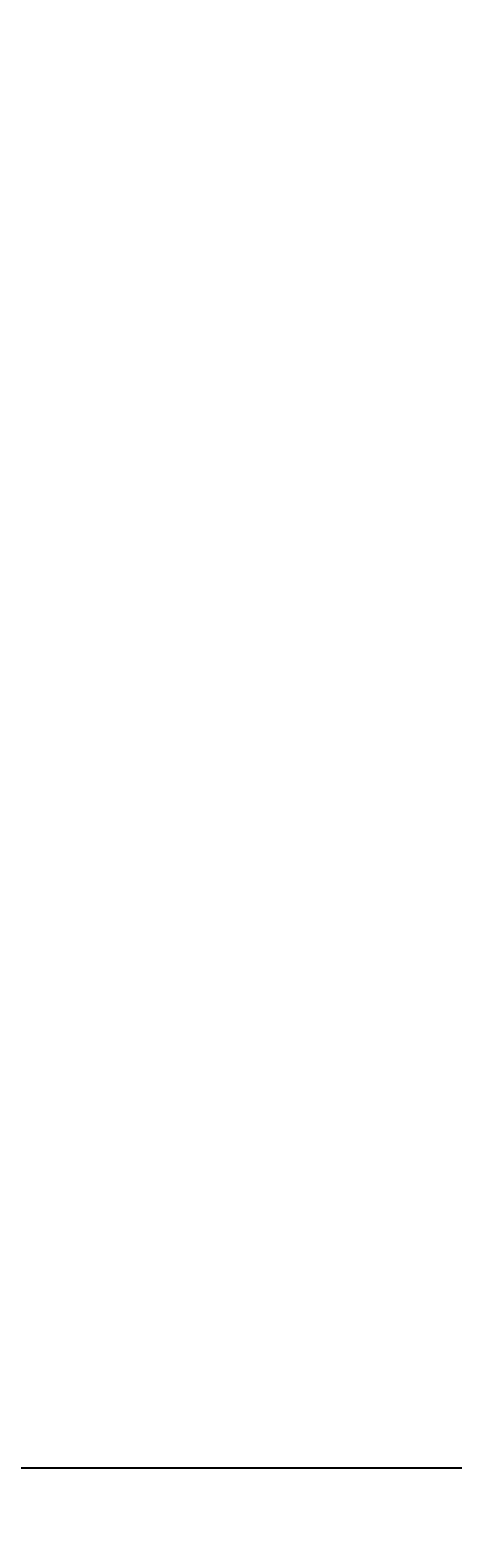
# Model space of a CAD drawing. Units: inches. Extents: x -61 to 1599, y -1316 to 257.
# Tile 11 of 204: x 200 to 222, y -1182 to -1105. Entities that reach past the tile are written whole.
import ezdxf

# ---------------------------------------------------------------- set-up
doc = ezdxf.new("R2010")
doc.units = ezdxf.units.IN
doc.header["$MEASUREMENT"] = 0
doc.layers.add('A-ANNO-DIMS', color=2, linetype='Continuous', lineweight=18)
doc.styles.get("Standard").update_dxf_attribs({"font": 'arial.ttf'})
doc.dimstyles.get("Standard").update_dxf_attribs({"dimtxt": 0.18, "dimasz": 0.18, "dimexe": 0.18, "dimexo": 0.0625, "dimgap": 0.09, "dimtad": 0, "dimtih": 1, "dimtoh": 1, "dimdec": 0, "dimzin": 0, "dimdsep": 46, "dimlunit": 3, "dimtxsty": 'Standard', "dimcen": 0.09, "dimadec": 0, "dimazin": 0, "dimtfac": 1, "dimtdec": 0, "dimtofl": 0, "dimtmove": 0, "dimatfit": 3, "dimfxl": 1, "dimtolj": 1, "dimtzin": 0, "dimarcsym": 0})

# ---------------------------------------------------------------- blocks, each defined once
blk = doc.blocks.new('*D687')
at = {"layer": 'A-ANNO-DIMS', "color": 0, "lineweight": -2, "transparency": 16777216}
for p, q in [((289.418, 181.677), (-61.077, 181.677)), ((-60.897, 181.497), (-60.897, -528.952)), ((-60.897, -1239.765), (-60.897, -529.316)), ((319.64, -1239.945), (-61.077, -1239.945))]:
    blk.add_line(p, q, dxfattribs=at)
at = {"layer": 'A-ANNO-DIMS', "color": 0, "transparency": 16777216}
for points in [[(-60.927, 181.497), (-60.867, 181.497), (-60.897, 181.677)], [(-60.927, -1239.765), (-60.867, -1239.765), (-60.897, -1239.945)]]:
    blk.add_solid(points, dxfattribs=at)
at = {"layer": 'DEFPOINTS', "color": 0, "transparency": 16777216}
for p in [(289.481, 181.677), (-60.897, -1239.945), (319.703, -1239.945)]:
    blk.add_point(p, dxfattribs=at)
at = {"layer": 'A-ANNO-DIMS', "color": 0, "transparency": 16777216, "insert": (-60.897, -529.134), "char_height": 0.18, "attachment_point": 5}
blk.add_mtext('\\A1;1421.6', dxfattribs=at)
blk = doc.blocks.new('*D696')
at = {"layer": 'A-ANNO-DIMS', "color": 0, "lineweight": -2, "transparency": 16777216}
for p, q in [((690.64, -873.169), (-61.077, -873.169)), ((-60.897, -873.349), (-60.897, -1025.799)), ((-60.897, -1178.613), (-60.897, -1026.163)), ((690.64, -1178.793), (-61.077, -1178.793))]:
    blk.add_line(p, q, dxfattribs=at)
at = {"layer": 'A-ANNO-DIMS', "color": 0, "transparency": 16777216}
for points in [[(-60.927, -873.349), (-60.867, -873.349), (-60.897, -873.169)], [(-60.927, -1178.613), (-60.867, -1178.613), (-60.897, -1178.793)]]:
    blk.add_solid(points, dxfattribs=at)
at = {"layer": 'DEFPOINTS', "color": 0, "transparency": 16777216}
for p in [(-60.897, -873.169), (690.703, -873.169), (690.703, -1178.793)]:
    blk.add_point(p, dxfattribs=at)
at = {"layer": 'A-ANNO-DIMS', "color": 0, "transparency": 16777216, "insert": (-60.897, -1025.981), "char_height": 0.18, "attachment_point": 5}
blk.add_mtext('\\A1;305.6', dxfattribs=at)

msp = doc.modelspace()

# ---------------------------------------------------------------- dimensions: what is measured, and where the dimension line sits
at = {"layer": 'A-ANNO-DIMS'}
for base, p1, p2, picture, middle in [((-60.8972, -1239.9446), (289.4807, 181.6771), (319.7028, -1239.9446), '*D687', (-60.8972, -529.1337)), ((-60.8972, -873.169), (690.7028, -1178.7933), (690.7028, -873.169), '*D696', (-60.8972, -1025.9812))]:
    dim = msp.add_linear_dim(base=base, p1=p1, p2=p2, angle=90, dimstyle='Standard', override={"dimdec": 1, "dimlfac": 1, "dimrnd": 0, "dimzin": 0, "dimdsep": 46, "dimlunit": 2}, dxfattribs=at)
    dim.commit()
    dim.dimension.update_dxf_attribs({"geometry": picture, "text_midpoint": middle})

doc.saveas('drawing.dxf')
